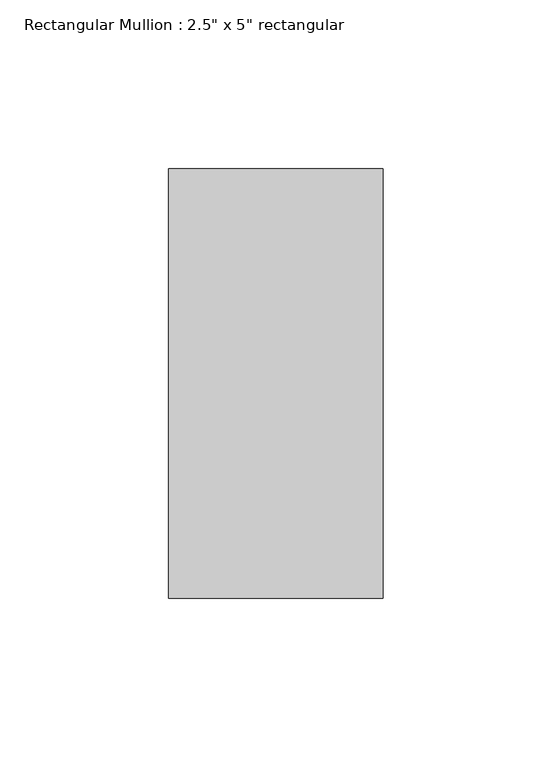
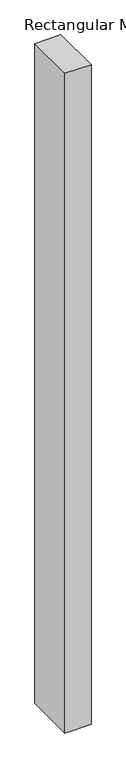
"""IFC4 building model written with IfcOpenShell, lengths in millimetres: member geometry."""

from ifc_helpers import new_model, si_unit, frame, origin, place, context, project, spatial, polyline, outline, extrude, source, transform, mapped, element, save


def member_145ad7ec(model_context):
    return source(origin(), model_context, "Body", "SweptSolid", [
        extrude(outline(polyline([(0.0, 63.5), (0.0, -63.5), (-63.5, -63.5), (-63.5, 63.5), (0.0, 63.5)])), frame((0.0, 0.0, -1700.4017583), z_axis=(0.0, 0.0, 1.0), x_axis=(1.0, 0.0, 0.0)), (0.0, 0.0, 1.0), 1700.4017583),
    ])


if __name__ == "__main__":
    model = new_model("IFC4")
    model_context = context("Model", 3, world=origin())
    ifc_project = project(units=[si_unit("LENGTHUNIT", "METRE", prefix="MILLI")], contexts=[model_context])
    site = spatial("IfcSite", under=ifc_project)
    building = spatial("IfcBuilding", under=site)
    placement = place(None, origin())
    member_shape = member_145ad7ec(model_context)
    element("IfcMember", 1, ObjectType="Rectangular Mullion : 2.5\" x 5\" rectangular", at=placement, inside=building, context=model_context, shape_type="MappedRepresentation", body=[
        mapped(member_shape, transform((0.0, 0.0, 0.0), x_axis=(1.0, 0.0, 0.0), y_axis=(0.0, 1.0, 0.0), z_axis=(0.0, 0.0, 1.0))),
    ])
    save(model, "model.ifc")

# Revit data of these elements
# Type "Rectangular Mullion : 2.5\" x 5\" rectangular"
#   built-in parameter 1007304 = 0.416667 (stored number, unit not read)
#   built-in parameter 1007301 = 0.104167 (stored number, unit not read)
#   built-in parameter 1007300 = 0.104167 (stored number, unit not read)
# Element 1 (IfcMember, "Rectangular Mullion : 2.5\" x 5\" rectangular")
#   Materials on its faces: "Aluminum"
# Materials
#   "Aluminum": class "Metal", colour RGB 247 247 247, transparency 0, Description = "Aluminum 6061", Cost = 0
